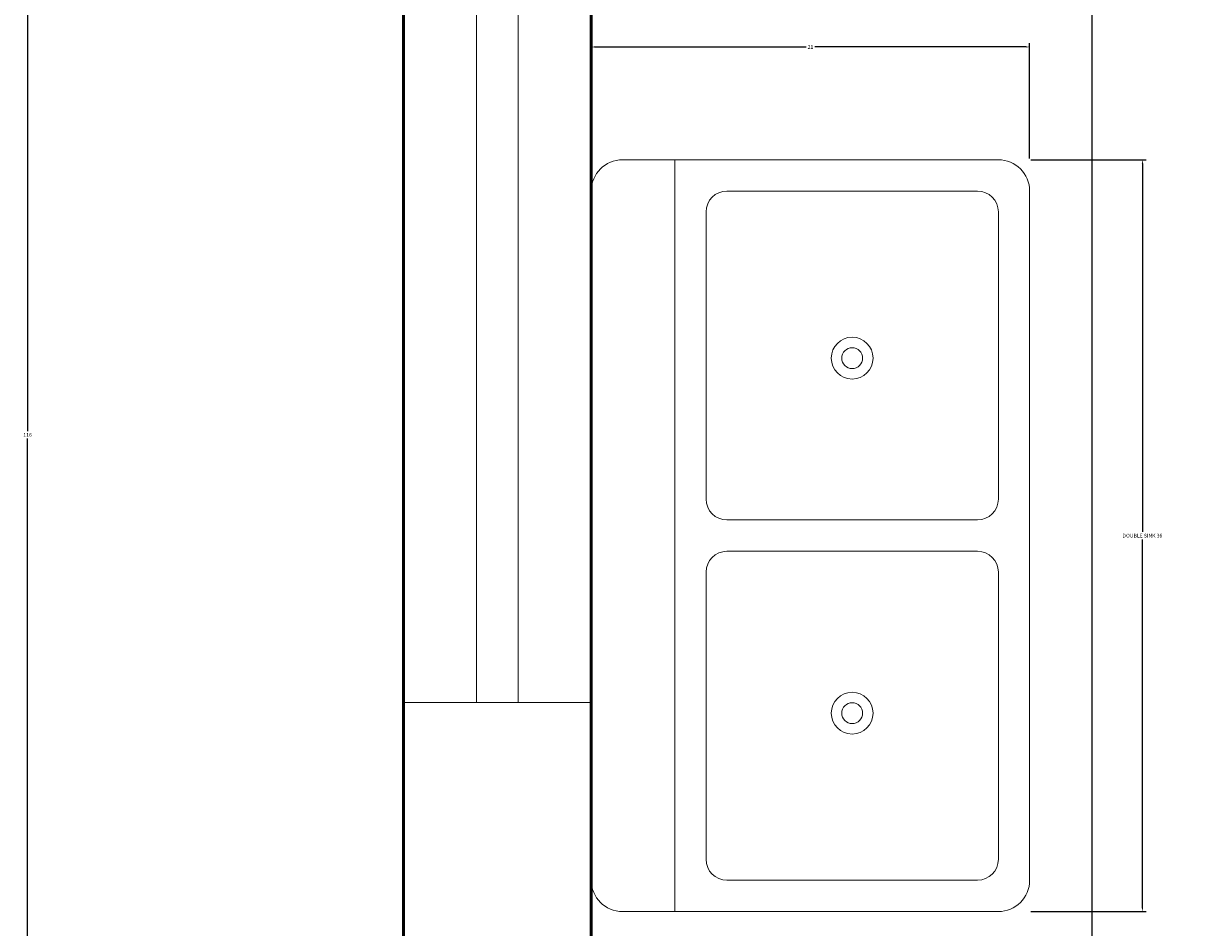
# Model space of a CAD drawing. Units: inches. Extents: x 2621 to 2849, y 2066 to 2463.
# Tile 8 of 28: x 2621 to 2676, y 2234 to 2277. Entities that reach past the tile are written whole.
import ezdxf

# ---------------------------------------------------------------- set-up
doc = ezdxf.new("R2010")
doc.units = ezdxf.units.IN
for name, color, linetype, lineweight in [('A-ANNO-DIMS', 2, 'Continuous', 18), ('A-FLOR-CASE', 9, 'Continuous', 25), ('A-FLOR-FIXT', 9, 'Continuous', 18), ('A-GLAZ', 4, 'Continuous', 18), ('A-WALL', 7, 'Continuous', 50)]:
    doc.layers.add(name, color=color, linetype=linetype, lineweight=lineweight)
doc.styles.get("Standard").update_dxf_attribs({"font": 'arial.ttf'})
doc.dimstyles.get("Standard").update_dxf_attribs({"dimtxt": 0.18, "dimasz": 0.18, "dimexe": 0.18, "dimexo": 0.0625, "dimgap": 0.09, "dimtad": 0, "dimtih": 1, "dimtoh": 1, "dimdec": 4, "dimzin": 0, "dimdsep": 46, "dimtxsty": 'Standard', "dimcen": 0.09, "dimadec": 0, "dimazin": 0, "dimtfac": 1, "dimtdec": 4, "dimtofl": 0, "dimtmove": 0, "dimatfit": 3, "dimfxl": 1, "dimtolj": 1, "dimtzin": 0, "dimarcsym": 0})

# ---------------------------------------------------------------- blocks, each defined once
blk = doc.blocks.new('Sink-double - 36 in top')
for p, q in [((-18, -4), (18, -4)), ((-0.75, -18.5), (-0.75, -6.5)), ((0.75, -6.5), (0.75, -18.5))]:
    blk.add_line(p, q)
for points in [[(-16.5, 0), (16.5, 0)], [(-18, -19.5), (-18, -1.5)], [(18, -1.5), (18, -19.5)], [(-15.5, -5.5), (-1.75, -5.5)], [(1.75, -5.5), (15.5, -5.5)], [(-16.5, -18.5), (-16.5, -6.5)], [(16.5, -6.5), (16.5, -18.5)], [(-1.75, -19.5), (-15.5, -19.5)], [(15.5, -19.5), (1.75, -19.5)], [(16.5, -21), (-16.5, -21)]]:
    blk.add_lwpolyline(points)
for centre, radius in [((-8.5, -12.5), 1), ((8.5, -12.5), 1), ((-8.5, -12.5), 0.5), ((8.5, -12.5), 0.5)]:
    blk.add_circle(centre, radius)
for centre, radius, start, end in [((-16.5, -1.5), 1.5, 90, 180), ((16.5, -1.5), 1.5, 0, 90), ((-15.5, -6.5), 1, 90, 180), ((-1.75, -6.5), 1, 0, 90), ((1.75, -6.5), 1, 90, 180), ((15.5, -6.5), 1, 0, 90), ((-15.5, -18.5), 1, 180, 270), ((-1.75, -18.5), 1, 270, 0), ((1.75, -18.5), 1, 180, 270), ((15.5, -18.5), 1, 270, 0), ((-16.5, -19.5), 1.5, 180, 270), ((16.5, -19.5), 1.5, 270, 0)]:
    blk.add_arc(centre, radius, start, end)
blk = doc.blocks.new('WIN-48IN')
for p, q in [((0, 5.5), (48, 5.5)), ((0, 3.5), (48, 3.5))]:
    blk.add_line(p, q)
for points in [[(0, 0), (0, 9)], [(48, 9), (48, 0)]]:
    blk.add_lwpolyline(points)
blk = doc.blocks.new('*D23')
at = {"layer": 'A-ANNO-DIMS', "color": 0, "lineweight": -2, "transparency": 16777216}
for p, q in [((2668.933, 2270.549), (2674.45, 2270.549)), ((2674.27, 2270.369), (2674.27, 2252.732)), ((2674.27, 2234.729), (2674.27, 2252.366)), ((2668.933, 2234.549), (2674.45, 2234.549))]:
    blk.add_line(p, q, dxfattribs=at)
at = {"layer": 'A-ANNO-DIMS', "color": 0, "transparency": 16777216}
for points in [[(2674.24, 2270.369), (2674.3, 2270.369), (2674.27, 2270.549)], [(2674.24, 2234.729), (2674.3, 2234.729), (2674.27, 2234.549)]]:
    blk.add_solid(points, dxfattribs=at)
at = {"layer": 'Defpoints', "color": 0, "transparency": 16777216}
for p in [(2668.87, 2270.549), (2674.27, 2270.549), (2668.87, 2234.549)]:
    blk.add_point(p, dxfattribs=at)
at = {"layer": 'A-ANNO-DIMS', "color": 0, "transparency": 16777216, "insert": (2674.27, 2252.549), "char_height": 0.18, "attachment_point": 5}
blk.add_mtext('\\A1;DOUBLE SINK 36', dxfattribs=at)
blk = doc.blocks.new('*D24')
at = {"layer": 'A-ANNO-DIMS', "color": 0, "lineweight": -2, "transparency": 16777216}
for p, q in [((2647.87, 2270.612), (2647.87, 2276.129)), ((2648.05, 2275.949), (2658.167, 2275.949)), ((2668.69, 2275.949), (2658.573, 2275.949)), ((2668.87, 2270.612), (2668.87, 2276.129))]:
    blk.add_line(p, q, dxfattribs=at)
at = {"layer": 'A-ANNO-DIMS', "color": 0, "transparency": 16777216}
for points in [[(2648.05, 2275.979), (2648.05, 2275.919), (2647.87, 2275.949)], [(2668.69, 2275.979), (2668.69, 2275.919), (2668.87, 2275.949)]]:
    blk.add_solid(points, dxfattribs=at)
at = {"layer": 'Defpoints', "color": 0, "transparency": 16777216}
for p in [(2647.87, 2275.949), (2647.87, 2270.549), (2668.87, 2270.549)]:
    blk.add_point(p, dxfattribs=at)
at = {"layer": 'A-ANNO-DIMS', "color": 0, "transparency": 16777216, "insert": (2658.37, 2275.949), "char_height": 0.18, "attachment_point": 5}
blk.add_mtext('\\A1;21', dxfattribs=at)
blk = doc.blocks.new('*D57')
at = {"layer": 'A-ANNO-DIMS', "color": 0, "lineweight": -2, "transparency": 16777216}
for p, q in [((2647.808, 2315.375), (2620.687, 2315.375)), ((2620.867, 2315.195), (2620.867, 2257.556)), ((2620.867, 2199.555), (2620.867, 2257.193)), ((2647.808, 2199.375), (2620.687, 2199.375))]:
    blk.add_line(p, q, dxfattribs=at)
at = {"layer": 'A-ANNO-DIMS', "color": 0, "transparency": 16777216}
for points in [[(2620.837, 2315.195), (2620.897, 2315.195), (2620.867, 2315.375)], [(2620.837, 2199.555), (2620.897, 2199.555), (2620.867, 2199.375)]]:
    blk.add_solid(points, dxfattribs=at)
at = {"layer": 'Defpoints', "color": 0, "transparency": 16777216}
for p in [(2620.867, 2315.375), (2647.87, 2315.375), (2647.87, 2199.375)]:
    blk.add_point(p, dxfattribs=at)
at = {"layer": 'A-ANNO-DIMS', "color": 0, "transparency": 16777216, "insert": (2620.867, 2257.375), "char_height": 0.18, "attachment_point": 5}
blk.add_mtext('\\A1;116', dxfattribs=at)

msp = doc.modelspace()

# ---------------------------------------------------------------- linework, layer by layer
at = {"layer": 'A-FLOR-CASE'}
msp.add_line((2671.8701, 2199.3746), (2671.8701, 2291.3746), dxfattribs=at)
at = {"layer": 'A-WALL'}
msp.add_line((2647.8701, 2199.3746), (2647.8701, 2315.3746), dxfattribs=at)
msp.add_lwpolyline([(2761.8701, 2084.3746), (2638.8701, 2084.3746), (2638.8701, 2444.3746), (2830.8701, 2444.3746), (2830.8701, 2084.3746), (2797.8701, 2084.3746)], dxfattribs=at)

# ---------------------------------------------------------------- block references
at = {"layer": 'A-FLOR-FIXT', "rotation": 90}
msp.add_blockref('Sink-double - 36 in top', (2647.8701, 2252.5492), dxfattribs=at)
at = {"layer": 'A-GLAZ', "rotation": 90.00000000000018}
msp.add_blockref('WIN-48IN', (2647.8701, 2244.5617), dxfattribs=at)

# ---------------------------------------------------------------- dimensions: what is measured, and where the dimension line sits
at = {"layer": 'A-ANNO-DIMS'}
for base, p1, p2, angle, picture, middle in [((2620.8666, 2315.3746), (2647.8701, 2199.3746), (2647.8701, 2315.3746), 90, '*D57', (2620.8666, 2257.3746)), ((2647.8701, 2275.9492), (2668.8701, 2270.5492), (2647.8701, 2270.5492), 180, '*D24', (2658.3701, 2275.9492))]:
    dim = msp.add_linear_dim(base=base, p1=p1, p2=p2, angle=angle, dimstyle='Standard', override={"dimdec": 0, "dimlfac": 1, "dimrnd": 0, "dimzin": 0, "dimdsep": 46, "dimlunit": 2}, dxfattribs=at)
    dim.commit()
    dim.dimension.update_dxf_attribs({"geometry": picture, "text_midpoint": middle})
dim = msp.add_linear_dim(base=(2674.2701, 2270.5492), p1=(2668.8701, 2234.5492), p2=(2668.8701, 2270.5492), angle=90, text='DOUBLE SINK <>', dimstyle='Standard', override={"dimdec": 0, "dimlfac": 1, "dimrnd": 0, "dimzin": 0, "dimdsep": 46, "dimlunit": 2}, dxfattribs=at)
dim.commit()
dim.dimension.update_dxf_attribs({"geometry": '*D23', "text_midpoint": (2674.2701, 2252.5492)})

doc.saveas('drawing.dxf')
